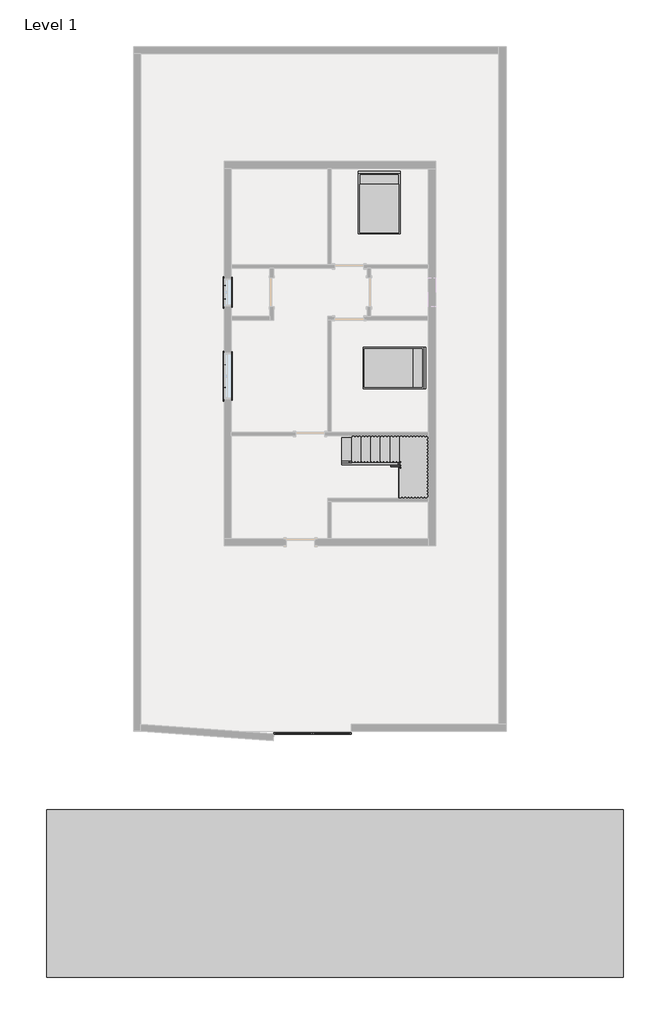
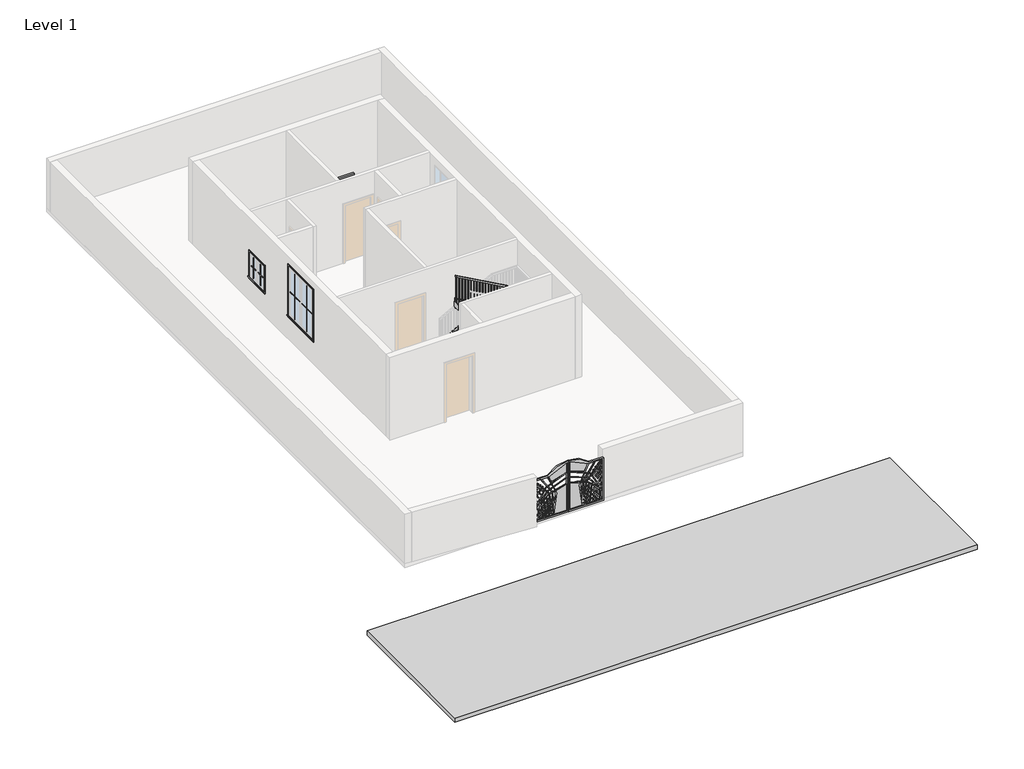
# One storey, part 2 of 2: 10 proxies, 6 members, 2 furniture elements, 1 railing, 1 stair flight.
"""IFC4 building model written with IfcOpenShell, lengths in millimetres."""

from ifc_helpers import new_model, si_unit, frame, origin, place, context, project, spatial, polyline, outline, extrude, faceted_brep, transform, mapped, element, save
from components import generic_models_6bc30956, generic_models_1_generic_models_1_070c5cf9, muntin_pattern_2x2_muntin_pattern_2x2_b3fe6957, muntin_pattern_2x2_muntin_pattern_2x2_3e0ecaf2, muntin_pattern_2x2_muntin_pattern_2x2_bff912c5, muntin_pattern_2x2_muntin_pattern_2x2_c2194282, trim_window_exterior_flat_with_sill_41619996, trim_window_exterior_flat_with_sill_e04b3088, trim_window_interior_flat_picture_frame_51c85655, trim_window_interior_flat_picture_frame_2a7685fe, bed_17739_bed_17739_15c61121, stair_flight_2c0e0b85

model = new_model("IFC4")

# Units and contexts
model_context = context("Model", 3, world=origin())
ifc_project = project(units=[si_unit("LENGTHUNIT", "METRE", prefix="MILLI")], contexts=[model_context])

# Site, building, storey
site = spatial("IfcSite", under=ifc_project)
building = spatial("IfcBuilding", under=site)
storey = spatial("IfcBuildingStorey", under=building, Name="Level 1", Elevation=0.0)

# Proxies
placement = place(None, origin())
generic_models_shape = generic_models_6bc30956(model_context)
element("IfcBuildingElementProxy", 1, Name="Generic Models", at=placement, inside=storey, context=model_context, shape_type="MappedRepresentation", body=[
    mapped(generic_models_shape, transform((-1820.2367916, -11481.1816344, 0.0), x_axis=(1.0, 0.0, 0.0), y_axis=(0.0, 1.0, 0.0), z_axis=(0.0, 0.0, 1.0))),
])
generic_models_1_generic_models_1_shape = generic_models_1_generic_models_1_070c5cf9(model_context)
element("IfcBuildingElementProxy", 2, Name="Generic Models 1 : Generic Models 1", ObjectType="Generic Models 1 : Generic Models 1", at=placement, inside=storey, context=model_context, shape_type="MappedRepresentation", body=[
    mapped(generic_models_1_generic_models_1_shape, transform((0.0, 0.0, 0.0), x_axis=(1.0, 0.0, 0.0), y_axis=(0.0, 1.0, 0.0), z_axis=(0.0, 0.0, 1.0))),
])
muntin_pattern_2x2_muntin_pattern_2x2_shape = muntin_pattern_2x2_muntin_pattern_2x2_b3fe6957(model_context)
element("IfcBuildingElementProxy", 3, Name="Muntin Pattern_2x2 : Muntin Pattern_2x2", ObjectType="Muntin Pattern_2x2 : Muntin Pattern_2x2", at=placement, inside=storey, context=model_context, shape_type="MappedRepresentation", body=[
    mapped(muntin_pattern_2x2_muntin_pattern_2x2_shape, transform((-4603.815747, 2266.9810985, 984.25), x_axis=(0.0, 1.0, 0.0), y_axis=(-1.0, 0.0, 0.0), z_axis=(0.0, 0.0, 1.0))),
])
muntin_pattern_2x2_muntin_pattern_2x2_2_shape = muntin_pattern_2x2_muntin_pattern_2x2_3e0ecaf2(model_context)
element("IfcBuildingElementProxy", 4, Name="Muntin Pattern_2x2 : Muntin Pattern_2x2", ObjectType="Muntin Pattern_2x2 : Muntin Pattern_2x2", at=placement, inside=storey, context=model_context, shape_type="MappedRepresentation", body=[
    mapped(muntin_pattern_2x2_muntin_pattern_2x2_2_shape, transform((-4603.815747, 2695.6060985, 984.25), x_axis=(0.0, -1.0, 0.0), y_axis=(1.0, 0.0, 0.0), z_axis=(0.0, 0.0, 1.0))),
])
muntin_pattern_2x2_muntin_pattern_2x2_3_shape = muntin_pattern_2x2_muntin_pattern_2x2_bff912c5(model_context)
element("IfcBuildingElementProxy", 5, Name="Muntin Pattern_2x2 : Muntin Pattern_2x2", ObjectType="Muntin Pattern_2x2 : Muntin Pattern_2x2", at=placement, inside=storey, context=model_context, shape_type="MappedRepresentation", body=[
    mapped(muntin_pattern_2x2_muntin_pattern_2x2_3_shape, transform((-4603.815747, -533.3689015, 984.25), x_axis=(0.0, 1.0, 0.0), y_axis=(-1.0, 0.0, 0.0), z_axis=(0.0, 0.0, 1.0))),
])
muntin_pattern_2x2_muntin_pattern_2x2_4_shape = muntin_pattern_2x2_muntin_pattern_2x2_c2194282(model_context)
element("IfcBuildingElementProxy", 6, Name="Muntin Pattern_2x2 : Muntin Pattern_2x2", ObjectType="Muntin Pattern_2x2 : Muntin Pattern_2x2", at=placement, inside=storey, context=model_context, shape_type="MappedRepresentation", body=[
    mapped(muntin_pattern_2x2_muntin_pattern_2x2_4_shape, transform((-4603.815747, 187.3560985, 984.25), x_axis=(0.0, -1.0, 0.0), y_axis=(1.0, 0.0, 0.0), z_axis=(0.0, 0.0, 1.0))),
])
trim_window_exterior_flat_with_sill_shape = trim_window_exterior_flat_with_sill_41619996(model_context)
element("IfcBuildingElementProxy", 7, Name="Trim-Window-Exterior-Flat : with Sill", ObjectType="Trim-Window-Exterior-Flat : with Sill", at=placement, inside=storey, context=model_context, shape_type="MappedRepresentation", body=[
    mapped(trim_window_exterior_flat_with_sill_shape, transform((-4613.340747, 2481.2935985, 1828.8), x_axis=(0.0, -1.0, 0.0), y_axis=(0.0, 0.0, 1.0), z_axis=(-1.0, 0.0, 0.0))),
])
trim_window_exterior_flat_with_sill_2_shape = trim_window_exterior_flat_with_sill_e04b3088(model_context)
element("IfcBuildingElementProxy", 8, Name="Trim-Window-Exterior-Flat : with Sill", ObjectType="Trim-Window-Exterior-Flat : with Sill", at=placement, inside=storey, context=model_context, shape_type="MappedRepresentation", body=[
    mapped(trim_window_exterior_flat_with_sill_2_shape, transform((-4613.340747, -173.0064015, 2743.2), x_axis=(0.0, -1.0, 0.0), y_axis=(0.0, 0.0, 1.0), z_axis=(-1.0, 0.0, 0.0))),
])
trim_window_interior_flat_picture_frame_shape = trim_window_interior_flat_picture_frame_51c85655(model_context)
element("IfcBuildingElementProxy", 9, Name="Trim-Window-Interior-Flat : Picture Frame", ObjectType="Trim-Window-Interior-Flat : Picture Frame", at=placement, inside=storey, context=model_context, shape_type="MappedRepresentation", body=[
    mapped(trim_window_interior_flat_picture_frame_shape, transform((-4384.740747, 2481.2935985, 1828.8), x_axis=(0.0, 1.0, 0.0), y_axis=(0.0, 0.0, 1.0), z_axis=(1.0, 0.0, 0.0))),
])
trim_window_interior_flat_picture_frame_2_shape = trim_window_interior_flat_picture_frame_2a7685fe(model_context)
element("IfcBuildingElementProxy", 10, Name="Trim-Window-Interior-Flat : Picture Frame", ObjectType="Trim-Window-Interior-Flat : Picture Frame", at=placement, inside=storey, context=model_context, shape_type="MappedRepresentation", body=[
    mapped(trim_window_interior_flat_picture_frame_2_shape, transform((-4384.740747, -173.0064015, 2743.2), x_axis=(0.0, 1.0, 0.0), y_axis=(0.0, 0.0, 1.0), z_axis=(1.0, 0.0, 0.0))),
])

# Furniture
bed_17739_bed_17739_shape = bed_17739_bed_17739_15c61121(model_context)
element("IfcFurniture", 11, ObjectType="Bed_17739 : Bed_17739", at=placement, inside=storey, context=model_context, shape_type="MappedRepresentation", body=[
    mapped(bed_17739_bed_17739_shape, transform((301.559253, 5300.6935985, 0.0), x_axis=(1.0, 0.0, 0.0), y_axis=(0.0, 1.0, 0.0), z_axis=(0.0, 0.0, 1.0))),
])
element("IfcFurniture", 12, ObjectType="Bed_17739 : Bed_17739", at=placement, inside=storey, context=model_context, shape_type="MappedRepresentation", body=[
    mapped(bed_17739_bed_17739_shape, transform((758.759253, 80.9935985, 0.0), x_axis=(0.0, -1.0, 0.0), y_axis=(1.0, 0.0, 0.0), z_axis=(0.0, 0.0, 1.0))),
])

# Members
element("IfcMember", 13, ObjectType="Stringer - 2\" Width", at=placement, inside=storey, context=model_context, shape_type="SweptSolid", body=[
    extrude(outline(polyline([(207.5983948, -879.540747), (0.0, -879.540747), (0.0, -625.5962442), (1261.5333333, 1645.1637558), (1261.5333333, 1017.5421424), (207.5983948, -879.540747)])), frame((0.0, -2065.3064015, 0.0), z_axis=(0.0, 1.0, 0.0), x_axis=(0.0, 0.0, 1.0)), (0.0, 0.0, 1.0), 50.8),
])
element("IfcMember", 14, ObjectType="Stringer - 2\" Width", at=placement, inside=storey, context=model_context, shape_type="SweptSolid", body=[
    extrude(outline(polyline([(1863.659253, -2014.5064015), (1914.459253, -2014.5064015), (1914.459253, -4046.5064015), (1863.659253, -4046.5064015), (1863.659253, -2014.5064015)])), frame((0.0, 0.0, 956.7333333), z_axis=(0.0, 0.0, 1.0), x_axis=(1.0, 0.0, 0.0)), (0.0, 0.0, 1.0), 304.8),
])
element("IfcMember", 15, ObjectType="Stringer - 2\" Width", at=placement, inside=storey, context=model_context, shape_type="SweptSolid", body=[
    extrude(outline(polyline([(956.7333333, 1734.4163636), (2408.9317281, -879.540747), (2060.253054, -879.540747), (956.7333333, 1106.7947502), (956.7333333, 1734.4163636)])), frame((0.0, -4097.3064015, 0.0), z_axis=(0.0, 1.0, 0.0), x_axis=(0.0, 0.0, 1.0)), (0.0, 0.0, 1.0), 50.8),
])
element("IfcMember", 16, ObjectType="Stringer - 2\" Width", at=placement, inside=storey, context=model_context, shape_type="SweptSolid", body=[
    extrude(outline(polyline([(207.5983948, -879.540747), (0.0, -879.540747), (0.0, -625.5962442), (846.6974984, 898.459253), (1195.3761726, 898.459253), (207.5983948, -879.540747)])), frame((0.0, -2979.7064015, 0.0), z_axis=(0.0, 1.0, 0.0), x_axis=(0.0, 0.0, 1.0)), (0.0, 0.0, 1.0), 50.8),
])
element("IfcMember", 17, ObjectType="Stringer - 2\" Width", at=placement, inside=storey, context=model_context, shape_type="SweptSolid", body=[
    extrude(outline(polyline([(898.459253, -2928.9064015), (949.259253, -2928.9064015), (949.259253, -3005.1064015), (898.459253, -3005.1064015), (898.459253, -2928.9064015)])), frame((0.0, 0.0, 956.7333333), z_axis=(0.0, 0.0, 1.0), x_axis=(1.0, 0.0, 0.0)), (0.0, 0.0, 1.0), 304.8),
])
element("IfcMember", 18, ObjectType="Stringer - 2\" Width", at=placement, inside=storey, context=model_context, shape_type="SweptSolid", body=[
    extrude(outline(polyline([(1044.253054, 949.259253), (1392.9317281, 949.259253), (2408.9317281, -879.540747), (2060.253054, -879.540747), (1044.253054, 949.259253)])), frame((0.0, -3055.9064015, 0.0), z_axis=(0.0, 1.0, 0.0), x_axis=(0.0, 0.0, 1.0)), (0.0, 0.0, 1.0), 50.8),
])

# Railing
element("IfcRailing", 19, ObjectType="Handrail - Rectangular", at=placement, inside=storey, context=model_context, shape_type="SolidModel", body=[
    faceted_brep([(-879.540747, -2878.1064015, 1083.7333333), (-879.540747, -2878.1064015, 1025.620221), (-879.540747, -2928.9064015, 1025.620221), (-879.540747, -2928.9064015, 1083.7333333), (873.059253, -2878.1064015, 2057.4), (923.859253, -2878.1064015, 2027.5091099), (923.859253, -2928.9064015, 2027.5091099), (873.059253, -2928.9064015, 2057.4), (873.059253, -2878.1064015, 2099.7333333), (923.859253, -2878.1064015, 2048.9333333), (923.859253, -2928.9064015, 2048.9333333), (873.059253, -2928.9064015, 2099.7333333), (1000.059253, -2878.1064015, 2099.7333333), (1000.059253, -2878.1064015, 2048.9333333), (949.259253, -2928.9064015, 2048.9333333), (949.259253, -2928.9064015, 2099.7333333), (1000.059253, -3005.1064015, 2099.7333333), (1000.059253, -3005.1064015, 2048.9333333), (949.259253, -3005.1064015, 2048.9333333), (949.259253, -3005.1064015, 2099.7333333), (1000.059253, -3055.9064015, 2099.7333333), (949.259253, -3055.9064015, 2099.7333333), (949.259253, -3106.7064015, 2048.9333333), (1000.059253, -3106.7064015, 2048.9333333)], [[[0, 1, 2, 3]], [[1, 0, 4, 5]], [[2, 1, 5, 6]], [[3, 2, 6, 7]], [[0, 3, 7, 4]], [[5, 4, 8, 9]], [[6, 5, 9, 10]], [[7, 6, 10, 11]], [[4, 7, 11, 8]], [[9, 8, 12, 13]], [[10, 9, 13, 14]], [[11, 10, 14, 15]], [[8, 11, 15, 12]], [[13, 12, 16, 17]], [[14, 13, 17, 18]], [[15, 14, 18, 19]], [[12, 15, 19, 16]], [[20, 21, 22, 23]], [[17, 16, 20, 23]], [[18, 17, 23, 22]], [[19, 18, 22, 21]], [[16, 19, 21, 20]]]),
    faceted_brep([(1000.059253, -3055.9064015, 2099.7333333), (1000.059253, -3106.7064015, 2048.9333333), (949.259253, -3106.7064015, 2048.9333333), (949.259253, -3055.9064015, 2099.7333333), (1000.059253, -3055.9064015, 2240.8444444), (949.259253, -3055.9064015, 2210.9535543), (949.259253, -3106.7064015, 2210.9535543), (1000.059253, -3106.7064015, 2240.8444444)], [[[0, 1, 2, 3]], [[4, 5, 6, 7]], [[1, 0, 4, 7]], [[2, 1, 7, 6]], [[3, 2, 6, 5]], [[0, 3, 5, 4]]]),
    faceted_brep([(1000.059253, -3106.7064015, 2240.8444444), (949.259253, -3106.7064015, 2210.9535543), (949.259253, -3055.9064015, 2210.9535543), (1000.059253, -3055.9064015, 2240.8444444), (-879.540747, -3106.7064015, 3285.0666667), (-879.540747, -3055.9064015, 3285.0666667), (-879.540747, -3055.9064015, 3226.9535543), (-879.540747, -3106.7064015, 3226.9535543)], [[[0, 1, 2, 3]], [[4, 5, 6, 7]], [[1, 0, 4, 7]], [[2, 1, 7, 6]], [[3, 2, 6, 5]], [[0, 3, 5, 4]]]),
    extrude(outline(polyline([(3207.5507765, -844.615747), (3218.1341099, -863.665747), (2201.3333333, -863.665747), (2201.3333333, -844.615747), (3207.5507765, -844.615747)])), frame((0.0, -3090.8314015, 0.0), z_axis=(0.0, 1.0, 0.0), x_axis=(0.0, 0.0, 1.0)), (0.0, 0.0, 1.0), 19.05),
    extrude(outline(polyline([(3151.1063321, -743.015747), (3161.6896654, -762.065747), (2201.3333333, -762.065747), (2201.3333333, -743.015747), (3151.1063321, -743.015747)])), frame((0.0, -3090.8314015, 0.0), z_axis=(0.0, 1.0, 0.0), x_axis=(0.0, 0.0, 1.0)), (0.0, 0.0, 1.0), 19.05),
    extrude(outline(polyline([(3094.6618876, -641.415747), (3105.245221, -660.465747), (2201.3333333, -660.465747), (2201.3333333, -641.415747), (3094.6618876, -641.415747)])), frame((0.0, -3090.8314015, 0.0), z_axis=(0.0, 1.0, 0.0), x_axis=(0.0, 0.0, 1.0)), (0.0, 0.0, 1.0), 19.05),
    extrude(outline(polyline([(3038.2174432, -539.815747), (3048.8007765, -558.865747), (2032.0, -558.865747), (2032.0, -539.815747), (3038.2174432, -539.815747)])), frame((0.0, -3090.8314015, 0.0), z_axis=(0.0, 1.0, 0.0), x_axis=(0.0, 0.0, 1.0)), (0.0, 0.0, 1.0), 19.05),
    extrude(outline(polyline([(2981.7729988, -438.215747), (2992.3563321, -457.265747), (2032.0, -457.265747), (2032.0, -438.215747), (2981.7729988, -438.215747)])), frame((0.0, -3090.8314015, 0.0), z_axis=(0.0, 1.0, 0.0), x_axis=(0.0, 0.0, 1.0)), (0.0, 0.0, 1.0), 19.05),
    extrude(outline(polyline([(2925.3285543, -336.615747), (2935.9118876, -355.665747), (2032.0, -355.665747), (2032.0, -336.615747), (2925.3285543, -336.615747)])), frame((0.0, -3090.8314015, 0.0), z_axis=(0.0, 1.0, 0.0), x_axis=(0.0, 0.0, 1.0)), (0.0, 0.0, 1.0), 19.05),
    extrude(outline(polyline([(2868.8841099, -235.015747), (2879.4674432, -254.065747), (1862.6666667, -254.065747), (1862.6666667, -235.015747), (2868.8841099, -235.015747)])), frame((0.0, -3090.8314015, 0.0), z_axis=(0.0, 1.0, 0.0), x_axis=(0.0, 0.0, 1.0)), (0.0, 0.0, 1.0), 19.05),
    extrude(outline(polyline([(2812.4396654, -133.415747), (2823.0229988, -152.465747), (1862.6666667, -152.465747), (1862.6666667, -133.415747), (2812.4396654, -133.415747)])), frame((0.0, -3090.8314015, 0.0), z_axis=(0.0, 1.0, 0.0), x_axis=(0.0, 0.0, 1.0)), (0.0, 0.0, 1.0), 19.05),
    extrude(outline(polyline([(2755.995221, -31.815747), (2766.5785543, -50.865747), (1862.6666667, -50.865747), (1862.6666667, -31.815747), (2755.995221, -31.815747)])), frame((0.0, -3090.8314015, 0.0), z_axis=(0.0, 1.0, 0.0), x_axis=(0.0, 0.0, 1.0)), (0.0, 0.0, 1.0), 19.05),
    extrude(outline(polyline([(2699.5507765, 69.784253), (2710.1341099, 50.734253), (1693.3333333, 50.734253), (1693.3333333, 69.784253), (2699.5507765, 69.784253)])), frame((0.0, -3090.8314015, 0.0), z_axis=(0.0, 1.0, 0.0), x_axis=(0.0, 0.0, 1.0)), (0.0, 0.0, 1.0), 19.05),
    extrude(outline(polyline([(2643.1063321, 171.384253), (2653.6896654, 152.334253), (1693.3333333, 152.334253), (1693.3333333, 171.384253), (2643.1063321, 171.384253)])), frame((0.0, -3090.8314015, 0.0), z_axis=(0.0, 1.0, 0.0), x_axis=(0.0, 0.0, 1.0)), (0.0, 0.0, 1.0), 19.05),
    extrude(outline(polyline([(2586.6618876, 272.984253), (2597.245221, 253.934253), (1693.3333333, 253.934253), (1693.3333333, 272.984253), (2586.6618876, 272.984253)])), frame((0.0, -3090.8314015, 0.0), z_axis=(0.0, 1.0, 0.0), x_axis=(0.0, 0.0, 1.0)), (0.0, 0.0, 1.0), 19.05),
    extrude(outline(polyline([(2530.2174432, 374.584253), (2540.8007765, 355.534253), (1524.0, 355.534253), (1524.0, 374.584253), (2530.2174432, 374.584253)])), frame((0.0, -3090.8314015, 0.0), z_axis=(0.0, 1.0, 0.0), x_axis=(0.0, 0.0, 1.0)), (0.0, 0.0, 1.0), 19.05),
    extrude(outline(polyline([(2473.7729988, 476.184253), (2484.3563321, 457.134253), (1524.0, 457.134253), (1524.0, 476.184253), (2473.7729988, 476.184253)])), frame((0.0, -3090.8314015, 0.0), z_axis=(0.0, 1.0, 0.0), x_axis=(0.0, 0.0, 1.0)), (0.0, 0.0, 1.0), 19.05),
    extrude(outline(polyline([(2417.3285543, 577.784253), (2427.9118876, 558.734253), (1524.0, 558.734253), (1524.0, 577.784253), (2417.3285543, 577.784253)])), frame((0.0, -3090.8314015, 0.0), z_axis=(0.0, 1.0, 0.0), x_axis=(0.0, 0.0, 1.0)), (0.0, 0.0, 1.0), 19.05),
    extrude(outline(polyline([(2360.8841099, 679.384253), (2371.4674432, 660.334253), (1354.6666667, 660.334253), (1354.6666667, 679.384253), (2360.8841099, 679.384253)])), frame((0.0, -3090.8314015, 0.0), z_axis=(0.0, 1.0, 0.0), x_axis=(0.0, 0.0, 1.0)), (0.0, 0.0, 1.0), 19.05),
    extrude(outline(polyline([(2304.4396654, 780.984253), (2315.0229988, 761.934253), (1354.6666667, 761.934253), (1354.6666667, 780.984253), (2304.4396654, 780.984253)])), frame((0.0, -3090.8314015, 0.0), z_axis=(0.0, 1.0, 0.0), x_axis=(0.0, 0.0, 1.0)), (0.0, 0.0, 1.0), 19.05),
    extrude(outline(polyline([(2247.995221, 882.584253), (2258.5785543, 863.534253), (1354.6666667, 863.534253), (1354.6666667, 882.584253), (2247.995221, 882.584253)])), frame((0.0, -3090.8314015, 0.0), z_axis=(0.0, 1.0, 0.0), x_axis=(0.0, 0.0, 1.0)), (0.0, 0.0, 1.0), 19.05),
    extrude(outline(polyline([(965.134253, -2995.5814015), (984.184253, -2995.5814015), (984.184253, -3014.6314015), (965.134253, -3014.6314015), (965.134253, -2995.5814015)])), frame((0.0, 0.0, 1185.3333333), z_axis=(0.0, 0.0, 1.0), x_axis=(1.0, 0.0, 0.0)), (0.0, 0.0, 1.0), 863.6),
    extrude(outline(polyline([(939.734253, -2913.0314015), (939.734253, -2893.9814015), (958.784253, -2893.9814015), (958.784253, -2913.0314015), (939.734253, -2913.0314015)])), frame((0.0, 0.0, 1185.3333333), z_axis=(0.0, 0.0, 1.0), x_axis=(1.0, 0.0, 0.0)), (0.0, 0.0, 1.0), 863.6),
    extrude(outline(polyline([(1990.4674432, 857.184253), (1979.8841099, 838.134253), (1016.0, 838.134253), (1016.0, 857.184253), (1990.4674432, 857.184253)])), frame((0.0, -2913.0314015, 0.0), z_axis=(0.0, 1.0, 0.0), x_axis=(0.0, 0.0, 1.0)), (0.0, 0.0, 1.0), 19.05),
    extrude(outline(polyline([(1934.0229988, 755.584253), (1923.4396654, 736.534253), (1016.0, 736.534253), (1016.0, 755.584253), (1934.0229988, 755.584253)])), frame((0.0, -2913.0314015, 0.0), z_axis=(0.0, 1.0, 0.0), x_axis=(0.0, 0.0, 1.0)), (0.0, 0.0, 1.0), 19.05),
    extrude(outline(polyline([(1877.5785543, 653.984253), (1866.995221, 634.934253), (1016.0, 634.934253), (1016.0, 653.984253), (1877.5785543, 653.984253)])), frame((0.0, -2913.0314015, 0.0), z_axis=(0.0, 1.0, 0.0), x_axis=(0.0, 0.0, 1.0)), (0.0, 0.0, 1.0), 19.05),
    extrude(outline(polyline([(1821.1341099, 552.384253), (1810.5507765, 533.334253), (846.6666667, 533.334253), (846.6666667, 552.384253), (1821.1341099, 552.384253)])), frame((0.0, -2913.0314015, 0.0), z_axis=(0.0, 1.0, 0.0), x_axis=(0.0, 0.0, 1.0)), (0.0, 0.0, 1.0), 19.05),
    extrude(outline(polyline([(1764.6896654, 450.784253), (1754.1063321, 431.734253), (846.6666667, 431.734253), (846.6666667, 450.784253), (1764.6896654, 450.784253)])), frame((0.0, -2913.0314015, 0.0), z_axis=(0.0, 1.0, 0.0), x_axis=(0.0, 0.0, 1.0)), (0.0, 0.0, 1.0), 19.05),
    extrude(outline(polyline([(1708.245221, 349.184253), (1697.6618876, 330.134253), (846.6666667, 330.134253), (846.6666667, 349.184253), (1708.245221, 349.184253)])), frame((0.0, -2913.0314015, 0.0), z_axis=(0.0, 1.0, 0.0), x_axis=(0.0, 0.0, 1.0)), (0.0, 0.0, 1.0), 19.05),
    extrude(outline(polyline([(1651.8007765, 247.584253), (1641.2174432, 228.534253), (677.3333333, 228.534253), (677.3333333, 247.584253), (1651.8007765, 247.584253)])), frame((0.0, -2913.0314015, 0.0), z_axis=(0.0, 1.0, 0.0), x_axis=(0.0, 0.0, 1.0)), (0.0, 0.0, 1.0), 19.05),
    extrude(outline(polyline([(1595.3563321, 145.984253), (1584.7729988, 126.934253), (677.3333333, 126.934253), (677.3333333, 145.984253), (1595.3563321, 145.984253)])), frame((0.0, -2913.0314015, 0.0), z_axis=(0.0, 1.0, 0.0), x_axis=(0.0, 0.0, 1.0)), (0.0, 0.0, 1.0), 19.05),
    extrude(outline(polyline([(1538.9118876, 44.384253), (1528.3285543, 25.334253), (677.3333333, 25.334253), (677.3333333, 44.384253), (1538.9118876, 44.384253)])), frame((0.0, -2913.0314015, 0.0), z_axis=(0.0, 1.0, 0.0), x_axis=(0.0, 0.0, 1.0)), (0.0, 0.0, 1.0), 19.05),
    extrude(outline(polyline([(1482.4674432, -57.215747), (1471.8841099, -76.265747), (508.0, -76.265747), (508.0, -57.215747), (1482.4674432, -57.215747)])), frame((0.0, -2913.0314015, 0.0), z_axis=(0.0, 1.0, 0.0), x_axis=(0.0, 0.0, 1.0)), (0.0, 0.0, 1.0), 19.05),
    extrude(outline(polyline([(1426.0229988, -158.815747), (1415.4396654, -177.865747), (508.0, -177.865747), (508.0, -158.815747), (1426.0229988, -158.815747)])), frame((0.0, -2913.0314015, 0.0), z_axis=(0.0, 1.0, 0.0), x_axis=(0.0, 0.0, 1.0)), (0.0, 0.0, 1.0), 19.05),
    extrude(outline(polyline([(1369.5785543, -260.415747), (1358.995221, -279.465747), (508.0, -279.465747), (508.0, -260.415747), (1369.5785543, -260.415747)])), frame((0.0, -2913.0314015, 0.0), z_axis=(0.0, 1.0, 0.0), x_axis=(0.0, 0.0, 1.0)), (0.0, 0.0, 1.0), 19.05),
    extrude(outline(polyline([(1313.1341099, -362.015747), (1302.5507765, -381.065747), (338.6666667, -381.065747), (338.6666667, -362.015747), (1313.1341099, -362.015747)])), frame((0.0, -2913.0314015, 0.0), z_axis=(0.0, 1.0, 0.0), x_axis=(0.0, 0.0, 1.0)), (0.0, 0.0, 1.0), 19.05),
    extrude(outline(polyline([(1256.6896654, -463.615747), (1246.1063321, -482.665747), (338.6666667, -482.665747), (338.6666667, -463.615747), (1256.6896654, -463.615747)])), frame((0.0, -2913.0314015, 0.0), z_axis=(0.0, 1.0, 0.0), x_axis=(0.0, 0.0, 1.0)), (0.0, 0.0, 1.0), 19.05),
    extrude(outline(polyline([(1200.245221, -565.215747), (1189.6618876, -584.265747), (338.6666667, -584.265747), (338.6666667, -565.215747), (1200.245221, -565.215747)])), frame((0.0, -2913.0314015, 0.0), z_axis=(0.0, 1.0, 0.0), x_axis=(0.0, 0.0, 1.0)), (0.0, 0.0, 1.0), 19.05),
    extrude(outline(polyline([(1143.8007765, -666.815747), (1133.2174432, -685.865747), (169.3333333, -685.865747), (169.3333333, -666.815747), (1143.8007765, -666.815747)])), frame((0.0, -2913.0314015, 0.0), z_axis=(0.0, 1.0, 0.0), x_axis=(0.0, 0.0, 1.0)), (0.0, 0.0, 1.0), 19.05),
    extrude(outline(polyline([(1087.3563321, -768.415747), (1076.7729988, -787.465747), (169.3333333, -787.465747), (169.3333333, -768.415747), (1087.3563321, -768.415747)])), frame((0.0, -2913.0314015, 0.0), z_axis=(0.0, 1.0, 0.0), x_axis=(0.0, 0.0, 1.0)), (0.0, 0.0, 1.0), 19.05),
    extrude(outline(polyline([(965.134253, -3071.7814015), (984.184253, -3071.7814015), (984.184253, -3090.8314015), (965.134253, -3090.8314015), (965.134253, -3071.7814015)])), frame((0.0, 0.0, 1185.3333333), z_axis=(0.0, 0.0, 1.0), x_axis=(1.0, 0.0, 0.0)), (0.0, 0.0, 1.0), 863.6),
    extrude(outline(polyline([(965.134253, -2913.0314015), (965.134253, -2893.9814015), (984.184253, -2893.9814015), (984.184253, -2913.0314015), (965.134253, -2913.0314015)])), frame((0.0, 0.0, 1185.3333333), z_axis=(0.0, 0.0, 1.0), x_axis=(1.0, 0.0, 0.0)), (0.0, 0.0, 1.0), 863.6),
    extrude(outline(polyline([(3216.370221, -860.490747), (3226.9535543, -879.540747), (2201.3333333, -879.540747), (2201.3333333, -860.490747), (3216.370221, -860.490747)])), frame((0.0, -3090.8314015, 0.0), z_axis=(0.0, 1.0, 0.0), x_axis=(0.0, 0.0, 1.0)), (0.0, 0.0, 1.0), 19.05),
    extrude(outline(polyline([(1036.2035543, -860.490747), (1025.620221, -879.540747), (169.3333333, -879.540747), (169.3333333, -860.490747), (1036.2035543, -860.490747)])), frame((0.0, -2913.0314015, 0.0), z_axis=(0.0, 1.0, 0.0), x_axis=(0.0, 0.0, 1.0)), (0.0, 0.0, 1.0), 19.05),
])

# Stair flight
stair_flight_shape = stair_flight_2c0e0b85(model_context)
element("IfcStairFlight", 20, ObjectType="2\" Tread 1\" Nosing 1/4\" Riser", at=placement, inside=storey, context=model_context, shape_type="MappedRepresentation", body=[
    mapped(stair_flight_shape, transform((0.0, 0.0, 0.0), x_axis=(1.0, 0.0, 0.0), y_axis=(0.0, 1.0, 0.0), z_axis=(0.0, 0.0, 1.0))),
])

save(model, "model.ifc")

# Revit data of these elements
# Type
#   m.s. sheet = none
#   2" x2" pipe = none
#   1"x1"pipe = none
#   Default Elevation = 0
# Type "Muntin Pattern_2x2 : Muntin Pattern_2x2"
#   Width [instance default] = 4' - 0"
#   Thickness = 0' - 0 1/2"
#   Height [instance default] = 4' - 0"
#   Distance = 0' - 0 3/4"
#   Interior Material [instance default] = none
#   Exterior Material [instance default] = none
#   Default Elevation = 0
# Type "Trim-Window-Exterior-Flat : with Sill"
#   Trim Width = 0' - 2 1/4"
#   Trim Thickness_Picture Frame = 0' - 1 1/4"
#   Trim Thickness_with Sill = 0' - 0 3/4"
#   Sill Thickness = 0' - 1 1/4"
#   Opening Width [instance default] = 2' - 0"
#   Opening Height [instance default] = 3' - 0"
#   Default Elevation = 4' - 0"
#   Sill = yes
#   Picture Frame = no
#   Trim Material [instance default] = none
# Type "Trim-Window-Interior-Flat : Picture Frame"
#   Trim Thickness_Picture Frame = 0' - 1 1/4"
#   Trim Width = 0' - 2 1/4"
#   Trim Thickness_with Sill = 0' - 0 3/4"
#   Sill Thickness = 0' - 1 1/4"
#   Opening Width [instance default] = 2' - 0"
#   Opening Height [instance default] = 3' - 0"
#   Default Elevation = 4' - 0"
#   Sill = no
#   Picture Frame = yes
#   Trim Material [instance default] = none
# Type "Bed_17739 : Bed_17739"
#   Default Elevation = 0
# Type "Handrail - Rectangular"
#   Assembly Code = "C2010400"
#   built-in parameter 1008612 = 0.0416667 (stored number, unit not read)
#   built-in parameter 1008611 = 0.0416667 (stored number, unit not read)
#   built-in parameter 1008609 = 0.333333 (stored number, unit not read)
#   built-in parameter 1008604 = 0.166667 (stored number, unit not read)
#   built-in parameter 1008603 = 0.166667 (stored number, unit not read)
#   Railing Height = 3' - 0"
#   built-in parameter 1008630 = 2
#   built-in parameter 1008610 = 2
#   built-in parameter 1008618 = Baluster - Square : 3/4"
# Element 1 (IfcBuildingElementProxy)
#   Phase Created = New Construction
#   Materials on its faces: "r1"
# Element 2 (IfcBuildingElementProxy, "Generic Models 1 : Generic Models 1")
#   Phase Created = New Construction
# Elements 3, 4 (IfcBuildingElementProxy, "Muntin Pattern_2x2 : Muntin Pattern_2x2")
#   Width = 0' - 11 5/8"
#   Height = 2' - 6 1/2"
#   Interior Material = Wood - Stained
#   Exterior Material = Clad - White
#   Phase Created = New Construction
#   Materials on its faces: "Clad - White", "Wood - Stained"
# Elements 5, 6 (IfcBuildingElementProxy, "Muntin Pattern_2x2 : Muntin Pattern_2x2")
#   Width = 1' - 11 1/8"
#   Height = 5' - 6 1/2"
#   Interior Material = Wood - Stained
#   Exterior Material = Clad - White
#   Phase Created = New Construction
#   Materials on its faces: "Clad - White", "Wood - Stained"
# Element 7 (IfcBuildingElementProxy, "Trim-Window-Exterior-Flat : with Sill")
#   Opening Width = 2' - 10"
#   Opening Height = 3' - 0"
#   Trim Material = Clad - White
#   Phase Created = New Construction
#   Materials on its faces: "Clad - White"
# Element 8 (IfcBuildingElementProxy, "Trim-Window-Exterior-Flat : with Sill")
#   Opening Width = 4' - 9"
#   Opening Height = 6' - 0"
#   Trim Material = Clad - White
#   Phase Created = New Construction
#   Materials on its faces: "Clad - White"
# Element 9 (IfcBuildingElementProxy, "Trim-Window-Interior-Flat : Picture Frame")
#   Opening Width = 2' - 10"
#   Opening Height = 3' - 0"
#   Trim Material = Wood - Stained
#   Phase Created = New Construction
#   Materials on its faces: "Wood - Stained"
# Element 10 (IfcBuildingElementProxy, "Trim-Window-Interior-Flat : Picture Frame")
#   Opening Width = 4' - 9"
#   Opening Height = 6' - 0"
#   Trim Material = Wood - Stained
#   Phase Created = New Construction
#   Materials on its faces: "Wood - Stained"
# Elements 11, 12 (IfcFurniture, "Bed_17739 : Bed_17739")
#   Phase Created = New Construction
#   Materials on its faces: "legs", "sheets", "bed frame", "Blanket"
# Elements 13, 14, 15, 16, 17, 18 (IfcMember, "Stringer - 2\" Width")
#   Phase Created = New Construction
# Element 19 (IfcRailing, "Handrail - Rectangular")
#   Phase Created = New Construction
# Element 20 (IfcStairFlight, "2\" Tread 1\" Nosing 1/4\" Riser")
#   Phase Created = New Construction
# Materials
#   "r1": class "Generic", colour RGB 120 120 120, transparency 0, Cost = 0
#   "Clad - White": class "Wood", colour RGB 242 242 238, transparency 0, Cost = 0
#   "Wood - Stained": class "Wood", colour RGB 224 178 126, transparency 0, Cost = 0
#   "legs": colour RGB 90 73 37, transparency 0, Cost = 0
#   "sheets": colour RGB 200 195 176, transparency 0, Cost = 0
#   "bed frame": colour RGB 90 73 37, transparency 0, Cost = 0
#   "Blanket": class "System", colour RGB 59 0 1, transparency 0, Cost = 0
